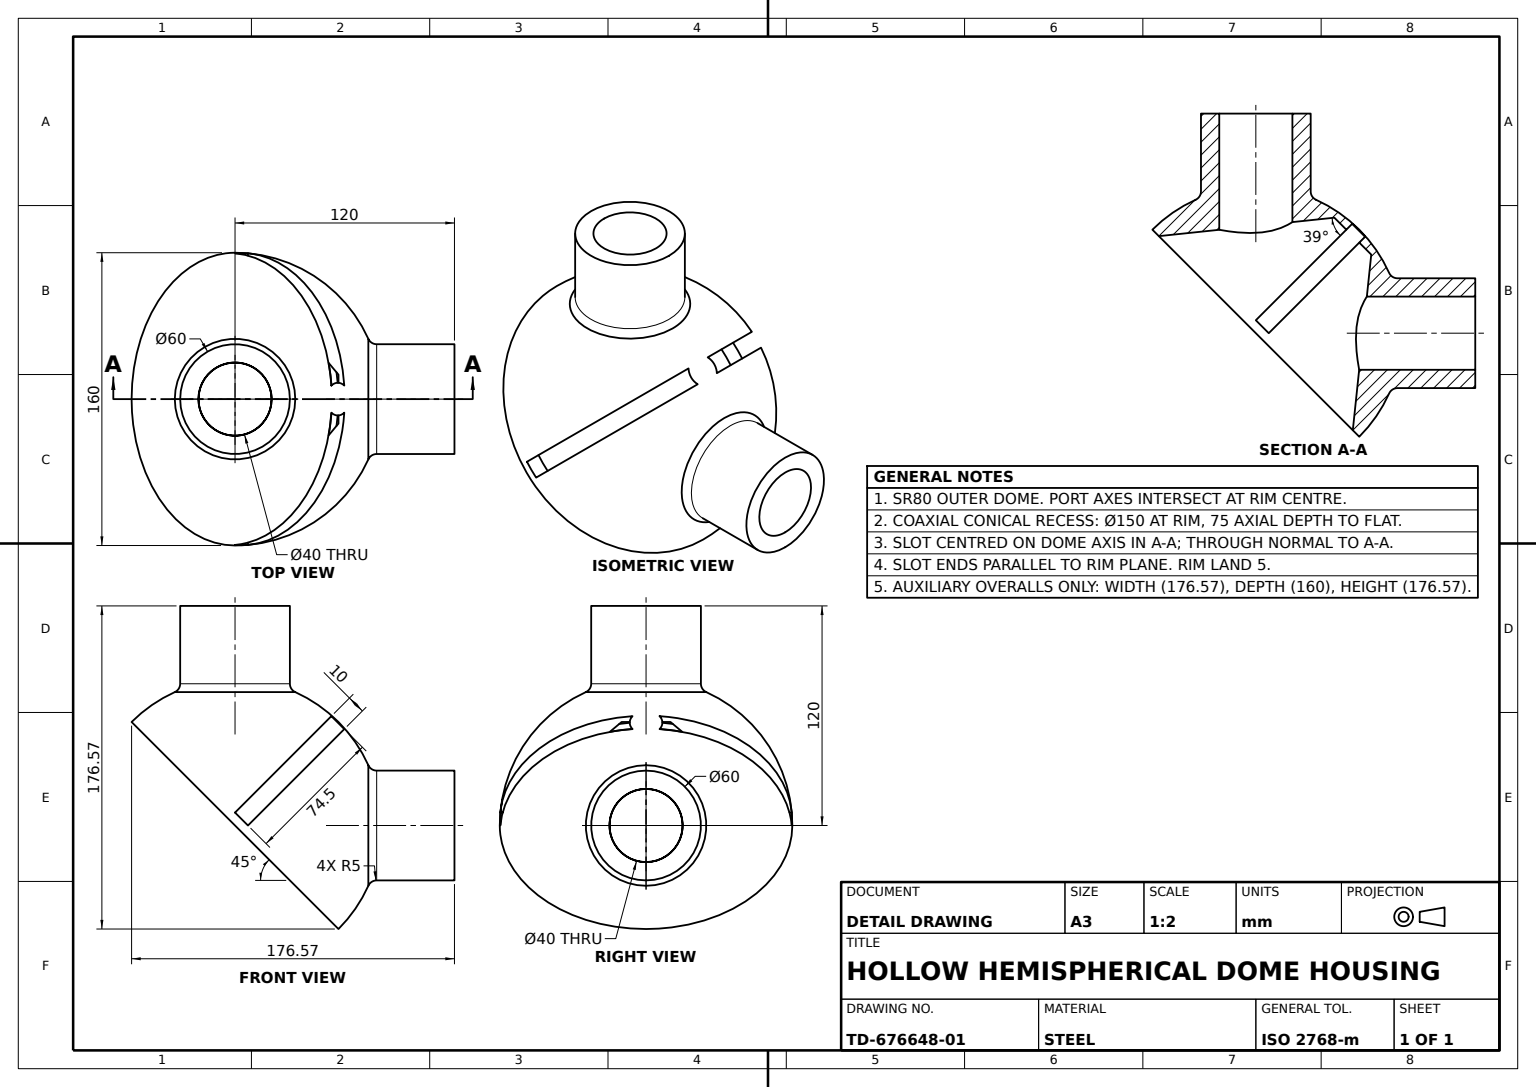
from build123d import *

# Parameters (mm, degrees)
DOME_SLOT_CUT_DEPTH = 105
ANGLED_CUT_SKETCH_R = 75
ANGLED_CUT_DEPTH    = 75
ANGLED_CUT_DRAFT    = -39
TUBE_BORE_SKETCH_R  = 20
TUBE_BORE_CUT_DEPTH = 75
TUBE_FILLET_R5_R    = 5


with BuildPart() as part:
    # Dome Profile Sketch → Dome R80 (revolve)
    with BuildSketch(Plane.XY):
        with BuildLine():
            Line((0, 0), (0, 80))
            ThreePointArc((0, 80), (56.568542495, 56.568542495), (80, 0))
            Line((80, 0), (0, 0))
        make_face()
    revolve(axis=Axis((0, 0, 0), (0, 1, 0)))

    # Dome Slot Sketch → Dome Slot Cut (cut, symmetric)
    with BuildSketch(Plane(origin=(0, 0, 0), x_dir=(0, 0, -1), z_dir=(1, 0, 0))):
        Polygon((5, 75), (5, 5), (-5, 5), (-5, 75), (-5, 78), (-5, 79), (-5, 79.5), (5, 79.5), (5, 78), align=None)
    extrude(amount=DOME_SLOT_CUT_DEPTH, both=True, mode=Mode.SUBTRACT)


with BuildPart() as angled_cut_tool:
    # Angled Cut Sketch → Angled Cut (with draft: the straight prism first)
    with BuildSketch(Plane.XZ):
        Circle(ANGLED_CUT_SKETCH_R)
    extrude(amount=-ANGLED_CUT_DEPTH)
    # Angled Cut: the draft: its side faces are tilted about the plane it starts from
    angled_cut_sides = [angled_cut_tool.faces().sort_by_distance(p)[0] for p in [
        (-75, 37.5, 0),
    ]]
    draft(angled_cut_sides, Plane.XZ, ANGLED_CUT_DRAFT)


with BuildPart() as part_1:
    add(part.part)

    # Angled Cut: cut by angled_cut_tool
    add(angled_cut_tool.part, mode=Mode.SUBTRACT)

    # Tube Boss Profile Sketch → Tube Boss (revolve)
    with BuildSketch(Plane(origin=(0, 0, 0), x_dir=(0, 0, -1), z_dir=(1, 0, 0))):
        Polygon((47.694291303, 47.694291303), (84.852813742, 84.852813742), (106.066017178, 63.639610307), (68.907494738, 26.481087867), (50.800202422, 44.588380184), align=None)
    tube_boss = revolve(axis=Axis((0, 47.694291303, -47.694291303), (0, 0.7071067811865478, -0.7071067811865474)))

    # Tube Bore Sketch → Tube Bore Cut (cut)
    with BuildSketch(Plane(origin=(0, 84.852813742, -84.852813742), x_dir=(1, 0, 0), z_dir=(0, 0.7071067811865477, -0.7071067811865475))):
        with Locations(Location((0, 0, 0), (0, 0, 270))):
            Circle(TUBE_BORE_SKETCH_R)
    tube_bore_cut = extrude(amount=-TUBE_BORE_CUT_DEPTH, mode=Mode.SUBTRACT)

    # Tube Bore Mirror: Tube Boss, Tube Bore Cut across plane
    add(tube_boss.mirror(Plane.XY))
    add(tube_bore_cut.mirror(Plane.XY), mode=Mode.SUBTRACT)

    # Tube Fillet R5
    tube_fillet_r5_edges = [part_1.edges().sort_by_distance(p)[0] for p in [
        (0, 73.653645844, -31.227238973),
        (0, 73.653645844, 31.227238973),
    ]]
    fillet(tube_fillet_r5_edges, radius=TUBE_FILLET_R5_R)


solid = part_1.part
